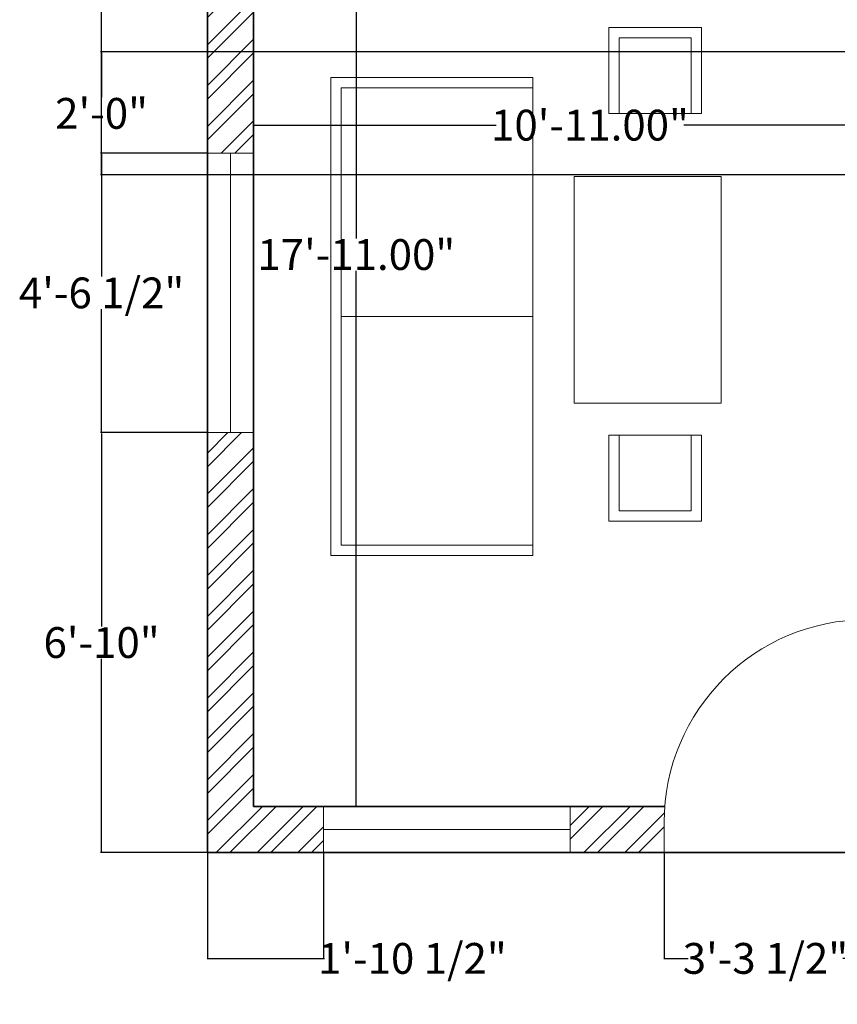
# Model space of a CAD drawing. Units: inches. Extents: x -20 to 887, y -143 to 410.
# Tile 1 of 5: x -20 to 139, y -11 to 180. Entities that reach past the tile are written whole.
import ezdxf

# ---------------------------------------------------------------- set-up
doc = ezdxf.new("R2010")
doc.units = ezdxf.units.IN
doc.header["$MEASUREMENT"] = 0
for name, color, linetype, lineweight in [('A-ANNO-DIMS', 2, 'Continuous', 18), ('A-DOOR', 3, 'Continuous', 18), ('A-FURN', 8, 'Continuous', 18), ('A-GLAZ', 4, 'Continuous', 18), ('A-WALL', 7, 'Continuous', 35), ('A-WALL-PATT', 8, 'Continuous', 13)]:
    doc.layers.add(name, color=color, linetype=linetype, lineweight=lineweight)
doc.styles.get("Standard").update_dxf_attribs({"font": 'arial.ttf'})
doc.dimstyles.get("Standard").update_dxf_attribs({"dimtxt": 6, "dimasz": 0.18, "dimexe": 0.18, "dimexo": 0.0625, "dimgap": 0.09, "dimtad": 0, "dimtih": 1, "dimtoh": 1, "dimzin": 0, "dimdsep": 46, "dimlunit": 3, "dimtxsty": 'Standard', "dimcen": 0.09, "dimadec": 0, "dimazin": 0, "dimtfac": 1, "dimtofl": 0, "dimtmove": 0, "dimatfit": 3, "dimfxl": 1, "dimtolj": 1, "dimtzin": 0, "dimarcsym": 0})

# ---------------------------------------------------------------- blocks, each defined once
blk = doc.blocks.new('*U2')
for p, q in [((0, 0), (0, -6)), ((40, 0), (40, -6))]:
    blk.add_line(p, q)
blk.add_lwpolyline([(0, 0), (0, 40), (1.75, 40), (1.75, 0)], close=True)
blk.add_arc((0, 0), 40, 0, 90)
blk = doc.blocks.new('*D11')
at = {"layer": 'A-ANNO-DIMS', "color": 0, "lineweight": -2, "transparency": 16777216}
for p, q in [((25.48, 242.13), (45.6, 242.13)), ((45.42, 241.95), (45.42, 137.79)), ((45.42, 27.31), (45.42, 131.48)), ((25.48, 27.13), (45.6, 27.13))]:
    blk.add_line(p, q, dxfattribs=at)
at = {"layer": 'A-ANNO-DIMS', "color": 0, "transparency": 16777216}
for points in [[(45.39, 241.95), (45.45, 241.95), (45.42, 242.13)], [(45.39, 27.31), (45.45, 27.31), (45.42, 27.13)]]:
    blk.add_solid(points, dxfattribs=at)
at = {"layer": 'Defpoints', "color": 0, "transparency": 16777216}
for p in [(25.42, 242.13), (25.42, 27.13), (45.42, 27.13)]:
    blk.add_point(p, dxfattribs=at)
at = {"layer": 'A-ANNO-DIMS', "color": 0, "transparency": 16777216, "insert": (45.42, 134.63), "char_height": 6, "attachment_point": 5}
blk.add_mtext('\\A1;17\'-11.00"', dxfattribs=at)
blk = doc.blocks.new('*D12')
at = {"layer": 'A-ANNO-DIMS', "color": 0, "lineweight": -2, "transparency": 16777216}
for p, q in [((25.42, 164.4), (25.42, 159.66)), ((156.42, 164.4), (156.42, 159.66)), ((25.6, 159.84), (72.65, 159.84)), ((156.24, 159.84), (109.19, 159.84))]:
    blk.add_line(p, q, dxfattribs=at)
at = {"layer": 'A-ANNO-DIMS', "color": 0, "transparency": 16777216}
for points in [[(25.6, 159.87), (25.6, 159.81), (25.42, 159.84)], [(156.24, 159.87), (156.24, 159.81), (156.42, 159.84)]]:
    blk.add_solid(points, dxfattribs=at)
at = {"layer": 'Defpoints', "color": 0, "transparency": 16777216}
for p in [(25.42, 164.46), (156.42, 164.46), (156.42, 159.84)]:
    blk.add_point(p, dxfattribs=at)
at = {"layer": 'A-ANNO-DIMS', "color": 0, "transparency": 16777216, "insert": (90.92, 159.84), "char_height": 6, "attachment_point": 5}
blk.add_mtext('\\A1;10\'-11.00"', dxfattribs=at)
blk = doc.blocks.new('WIN-48IN-9IN-WALL')
for p, q in [((9, 48), (0, 48)), ((4.5, 0), (4.5, 48)), ((9, 0), (0, 0))]:
    blk.add_line(p, q)
blk = doc.blocks.new('*D53')
at = {"layer": 'A-ANNO-DIMS', "color": 0, "lineweight": -2, "transparency": 16777216}
for p, q in [((16.42, 18.07), (16.42, -2.65)), ((39.06, 18.07), (39.06, -2.65)), ((16.6, -2.47), (38.88, -2.47)), ((39.06, -2.47), (39.24, -2.47))]:
    blk.add_line(p, q, dxfattribs=at)
at = {"layer": 'A-ANNO-DIMS', "color": 0, "transparency": 16777216}
for points in [[(16.6, -2.44), (16.6, -2.5), (16.42, -2.47)], [(38.88, -2.44), (38.88, -2.5), (39.06, -2.47)]]:
    blk.add_solid(points, dxfattribs=at)
at = {"layer": 'Defpoints', "color": 0, "transparency": 16777216}
for p in [(16.42, 18.13), (39.06, 18.13), (39.06, -2.47)]:
    blk.add_point(p, dxfattribs=at)
at = {"layer": 'A-ANNO-DIMS', "color": 0, "transparency": 16777216, "insert": (56.34, -2.47), "char_height": 6, "attachment_point": 5}
blk.add_mtext('\\A1;1\'-10 1/2"', dxfattribs=at)
blk = doc.blocks.new('*D54')
at = {"layer": 'A-ANNO-DIMS', "color": 0, "lineweight": -2, "transparency": 16777216}
for p, q in [((105.35, 18.07), (105.35, -2.65)), ((144.81, 18.07), (144.81, -2.65)), ((105.53, -2.47), (110.03, -2.47)), ((144.63, -2.47), (140.13, -2.47))]:
    blk.add_line(p, q, dxfattribs=at)
at = {"layer": 'A-ANNO-DIMS', "color": 0, "transparency": 16777216}
for points in [[(105.53, -2.44), (105.53, -2.5), (105.35, -2.47)], [(144.63, -2.44), (144.63, -2.5), (144.81, -2.47)]]:
    blk.add_solid(points, dxfattribs=at)
at = {"layer": 'Defpoints', "color": 0, "transparency": 16777216}
for p in [(105.35, 18.13), (144.81, 18.13), (144.81, -2.47)]:
    blk.add_point(p, dxfattribs=at)
at = {"layer": 'A-ANNO-DIMS', "color": 0, "transparency": 16777216, "insert": (125.08, -2.47), "char_height": 6, "attachment_point": 5}
blk.add_mtext('\\A1;3\'-3 1/2"', dxfattribs=at)
blk = doc.blocks.new('*D58')
at = {"layer": 'A-ANNO-DIMS', "color": 0, "lineweight": -2, "transparency": 16777216}
for p, q in [((16.35, 99.96), (-4.36, 99.96)), ((-4.18, 99.78), (-4.18, 62.2)), ((-4.18, 18.31), (-4.18, 55.89)), ((16.35, 18.13), (-4.36, 18.13))]:
    blk.add_line(p, q, dxfattribs=at)
at = {"layer": 'A-ANNO-DIMS', "color": 0, "transparency": 16777216}
for points in [[(-4.21, 99.78), (-4.15, 99.78), (-4.18, 99.96)], [(-4.21, 18.31), (-4.15, 18.31), (-4.18, 18.13)]]:
    blk.add_solid(points, dxfattribs=at)
at = {"layer": 'Defpoints', "color": 0, "transparency": 16777216}
for p in [(-4.18, 99.96), (16.42, 99.96), (16.42, 18.13)]:
    blk.add_point(p, dxfattribs=at)
at = {"layer": 'A-ANNO-DIMS', "color": 0, "transparency": 16777216, "insert": (-4.18, 59.05), "char_height": 6, "attachment_point": 5}
blk.add_mtext('\\A1;6\'-10"', dxfattribs=at)
blk = doc.blocks.new('*D59')
at = {"layer": 'A-ANNO-DIMS', "color": 0, "lineweight": -2, "transparency": 16777216}
for p, q in [((16.35, 154.36), (-4.36, 154.36)), ((-4.18, 154.18), (-4.18, 130.35)), ((-4.18, 100.14), (-4.18, 123.97)), ((16.35, 99.96), (-4.36, 99.96))]:
    blk.add_line(p, q, dxfattribs=at)
at = {"layer": 'A-ANNO-DIMS', "color": 0, "transparency": 16777216}
for points in [[(-4.21, 154.18), (-4.15, 154.18), (-4.18, 154.36)], [(-4.21, 100.14), (-4.15, 100.14), (-4.18, 99.96)]]:
    blk.add_solid(points, dxfattribs=at)
at = {"layer": 'Defpoints', "color": 0, "transparency": 16777216}
for p in [(-4.18, 154.36), (16.42, 154.36), (16.42, 99.96)]:
    blk.add_point(p, dxfattribs=at)
at = {"layer": 'A-ANNO-DIMS', "color": 0, "transparency": 16777216, "insert": (-4.18, 127.16), "char_height": 6, "attachment_point": 5}
blk.add_mtext('\\A1;4\'-6 1/2"', dxfattribs=at)
blk = doc.blocks.new('*D60')
at = {"layer": 'A-ANNO-DIMS', "color": 0, "lineweight": -2, "transparency": 16777216}
for p, q in [((16.35, 276.44), (-4.36, 276.44)), ((-4.18, 276.26), (-4.18, 218.55)), ((-4.18, 154.54), (-4.18, 212.25)), ((16.35, 154.36), (-4.36, 154.36))]:
    blk.add_line(p, q, dxfattribs=at)
at = {"layer": 'A-ANNO-DIMS', "color": 0, "transparency": 16777216}
for points in [[(-4.21, 276.26), (-4.15, 276.26), (-4.18, 276.44)], [(-4.21, 154.54), (-4.15, 154.54), (-4.18, 154.36)]]:
    blk.add_solid(points, dxfattribs=at)
at = {"layer": 'Defpoints', "color": 0, "transparency": 16777216}
for p in [(-4.18, 276.44), (16.42, 276.44), (16.42, 154.36)]:
    blk.add_point(p, dxfattribs=at)
at = {"layer": 'A-ANNO-DIMS', "color": 0, "transparency": 16777216, "insert": (-4.18, 215.4), "char_height": 6, "attachment_point": 5}
blk.add_mtext('\\A1;10\'-2"', dxfattribs=at)
blk = doc.blocks.new('*D68')
at = {"layer": 'A-ANNO-DIMS', "color": 0, "lineweight": -2, "transparency": 16777216}
for p, q in [((197.32, 174.13), (-4.36, 174.13)), ((-4.18, 173.95), (-4.18, 165.29)), ((-4.18, 150.31), (-4.18, 158.98)), ((197.32, 150.13), (-4.36, 150.13))]:
    blk.add_line(p, q, dxfattribs=at)
at = {"layer": 'A-ANNO-DIMS', "color": 0, "transparency": 16777216}
for points in [[(-4.21, 173.95), (-4.15, 173.95), (-4.18, 174.13)], [(-4.21, 150.31), (-4.15, 150.31), (-4.18, 150.13)]]:
    blk.add_solid(points, dxfattribs=at)
at = {"layer": 'Defpoints', "color": 0, "transparency": 16777216}
for p in [(197.38, 174.13), (-4.18, 150.13), (197.38, 150.13)]:
    blk.add_point(p, dxfattribs=at)
at = {"layer": 'A-ANNO-DIMS', "color": 0, "transparency": 16777216, "insert": (-4.18, 162.13), "char_height": 6, "attachment_point": 5}
blk.add_mtext('\\A1;2\'-0"', dxfattribs=at)

msp = doc.modelspace()

# ---------------------------------------------------------------- hatches: boundary and pattern name
at = {"layer": 'A-WALL-PATT'}
h = msp.add_hatch(dxfattribs=at)
h.set_pattern_fill('ANSI32', color=256, scale=15)
h.paths.add_polyline_path([(25.417, 242.135), (120.561, 242.135), (120.561, 246.163, -0.0277279), (120.726, 249.135), (25.417, 249.135), (25.417, 276.435), (16.417, 276.435), (16.417, 154.363), (25.417, 154.363)])
h = msp.add_hatch(dxfattribs=at)
h.set_pattern_fill('ANSI32', color=256, scale=15)
h.paths.add_polyline_path([(39.057, 27.135), (25.417, 27.135), (25.417, 99.962), (16.417, 99.962), (16.417, 18.135), (39.057, 18.135)])
h = msp.add_hatch(dxfattribs=at)
h.set_pattern_fill('ANSI32', color=256, scale=15)
h.paths.add_polyline_path([(105.35, 24.054, -0.0195413), (105.47, 27.135), (87.057, 27.135), (87.057, 18.135), (105.35, 18.135)])

# ---------------------------------------------------------------- linework, layer by layer
at = {"layer": 'A-FURN'}
msp.add_line((42.449, 122.573), (79.795, 122.573), dxfattribs=at)
for points in [[(94.565, 178.868), (112.618, 178.868), (112.618, 162.089), (94.565, 162.089)], [(40.449, 169.114), (79.795, 169.114), (79.795, 76.033), (40.449, 76.033)], [(87.837, 149.817), (116.477, 149.817), (116.477, 105.684), (87.837, 105.684)], [(94.565, 99.473), (112.618, 99.473), (112.618, 82.694), (94.565, 82.694)]]:
    msp.add_lwpolyline(points, close=True, dxfattribs=at)
for points in [[(96.565, 162.089), (96.565, 176.868), (110.618, 176.868), (110.618, 162.089)], [(79.795, 78.033), (42.449, 78.033), (42.449, 167.114), (79.795, 167.114)], [(110.618, 99.473), (110.618, 84.694), (96.565, 84.694), (96.565, 99.473)]]:
    msp.add_lwpolyline(points, dxfattribs=at)
at = {"layer": 'A-GLAZ'}
for p, q in [((16.417, 154.363), (25.417, 154.363)), ((20.917, 154.363), (20.917, 99.962)), ((16.417, 99.962), (25.417, 99.962))]:
    msp.add_line(p, q, dxfattribs=at)
at = {"layer": 'A-WALL'}
msp.add_lwpolyline([(16.417, 18.135), (292.417, 18.135), (292.417, 378.135), (16.417, 378.135)], close=True, dxfattribs=at)
for points in [[(25.417, 242.135), (25.417, 27.135)], [(25.417, 27.135), (105.47, 27.135)]]:
    msp.add_lwpolyline(points, dxfattribs=at)

# ---------------------------------------------------------------- block references
at = {"layer": 'A-DOOR', "xscale": -0.9865145828543779, "yscale": 0.9865145828543779, "zscale": 0.9865145828543779}
msp.add_blockref('*U2', (144.81, 24.054), dxfattribs=at)
at = {"layer": 'A-GLAZ', "rotation": 270.0000000000001}
msp.add_blockref('WIN-48IN-9IN-WALL', (39.057, 27.134), dxfattribs=at)

# ---------------------------------------------------------------- dimensions: what is measured, and where the dimension line sits
at = {"layer": 'A-ANNO-DIMS'}
for base, p1, p2, override, picture, middle in [((-4.183, 276.435), (16.417, 154.363), (16.417, 276.435), {"dimdec": 1, "dimlfac": 1, "dimrnd": 0, "dimzin": 1, "dimdsep": 46, "dimlunit": 4, "dimfrac": 2}, '*D60', (-4.183, 215.399)), ((45.415, 27.135), (25.417, 242.135), (25.417, 27.135), {"dimclrd": 0, "dimclre": 0, "dimclrt": 0}, '*D11', (45.415, 134.635)), ((-4.183, 150.135), (197.379, 174.135), (197.379, 150.135), {"dimdec": 1, "dimlfac": 1, "dimrnd": 0, "dimzin": 1, "dimdsep": 46, "dimlunit": 4, "dimfrac": 2}, '*D68', (-4.183, 162.135)), ((-4.183, 154.363), (16.417, 99.962), (16.417, 154.363), {"dimdec": 1, "dimlfac": 1, "dimrnd": 0, "dimzin": 1, "dimdsep": 46, "dimlunit": 4, "dimfrac": 2}, '*D59', (-4.183, 127.163)), ((-4.183, 99.962), (16.417, 18.135), (16.417, 99.962), {"dimdec": 1, "dimlfac": 1, "dimrnd": 0, "dimzin": 1, "dimdsep": 46, "dimlunit": 4, "dimfrac": 2}, '*D58', (-4.183, 59.048))]:
    dim = msp.add_linear_dim(base=base, p1=p1, p2=p2, angle=90, dimstyle='Standard', override=override, dxfattribs=at)
    dim.commit()
    dim.dimension.update_dxf_attribs({"geometry": picture, "text_midpoint": middle})
for base, p1, p2, override, picture, middle in [((156.417, 159.836), (25.417, 164.461), (156.417, 164.461), {"dimclrd": 0, "dimclre": 0, "dimclrt": 0}, '*D12', (90.917, 159.836)), ((39.057, -2.465), (16.417, 18.135), (39.057, 18.135), {"dimdec": 1, "dimlfac": 1, "dimrnd": 0, "dimzin": 1, "dimdsep": 46, "dimlunit": 4, "dimfrac": 2}, '*D53', (56.341, -2.465)), ((144.81, -2.465), (105.35, 18.135), (144.81, 18.135), {"dimdec": 1, "dimlfac": 1, "dimrnd": 0, "dimzin": 1, "dimdsep": 46, "dimlunit": 4, "dimfrac": 2}, '*D54', (125.08, -2.465))]:
    dim = msp.add_linear_dim(base=base, p1=p1, p2=p2, dimstyle='Standard', override=override, dxfattribs=at)
    dim.commit()
    dim.dimension.update_dxf_attribs({"geometry": picture, "text_midpoint": middle})

doc.saveas('drawing.dxf')
